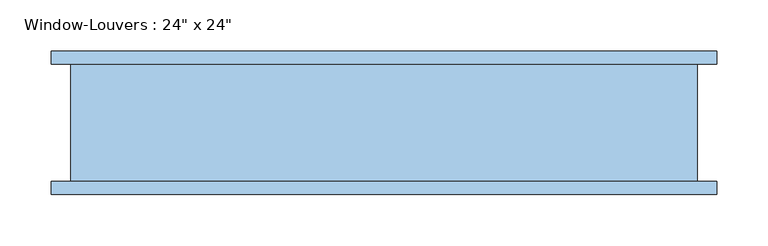
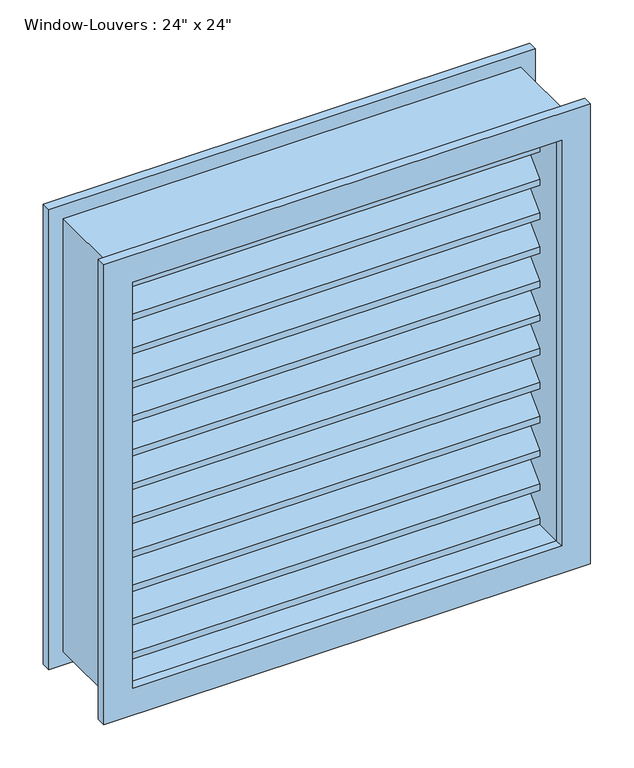
"""IFC4 building model written with IfcOpenShell, lengths in millimetres: window geometry."""

from ifc_helpers import new_model, si_unit, frame, origin, place, context, project, spatial, polyline, outline, extrude, source, transform, mapped, element, save


def window_d39e7ecb(model_context):
    return source(origin(), model_context, "Body", "SweptSolid", [
        extrude(outline(polyline([(50.8, 1419.1754778), (50.8, 1410.1952217), (12.7, 1448.2952217), (-25.4, 1410.1952217), (-25.4, 1419.1754778), (12.7, 1457.2754778), (50.8, 1419.1754778)])), frame((-285.75, 0.0, 0.0), z_axis=(1.0, 0.0, 0.0), x_axis=(0.0, 1.0, 0.0)), (0.0, 0.0, 1.0), 571.5),
        extrude(outline(polyline([(50.8, 1371.5009557), (50.8, 1362.5206995), (12.7, 1400.6206995), (-25.4, 1362.5206995), (-25.4, 1371.5009557), (12.7, 1409.6009557), (50.8, 1371.5009557)])), frame((-285.75, 0.0, 0.0), z_axis=(1.0, 0.0, 0.0), x_axis=(0.0, 1.0, 0.0)), (0.0, 0.0, 1.0), 571.5),
        extrude(outline(polyline([(50.8, 1323.8264335), (50.8, 1314.8461774), (12.7, 1352.9461774), (-25.4, 1314.8461774), (-25.4, 1323.8264335), (12.7, 1361.9264335), (50.8, 1323.8264335)])), frame((-285.75, 0.0, 0.0), z_axis=(1.0, 0.0, 0.0), x_axis=(0.0, 1.0, 0.0)), (0.0, 0.0, 1.0), 571.5),
        extrude(outline(polyline([(50.8, 1276.1519113), (50.8, 1267.1716552), (12.7, 1305.2716552), (-25.4, 1267.1716552), (-25.4, 1276.1519113), (12.7, 1314.2519113), (50.8, 1276.1519113)])), frame((-285.75, 0.0, 0.0), z_axis=(1.0, 0.0, 0.0), x_axis=(0.0, 1.0, 0.0)), (0.0, 0.0, 1.0), 571.5),
        extrude(outline(polyline([(50.8, 1228.4773891), (50.8, 1219.497133), (12.7, 1257.597133), (-25.4, 1219.497133), (-25.4, 1228.4773891), (12.7, 1266.5773891), (50.8, 1228.4773891)])), frame((-285.75, 0.0, 0.0), z_axis=(1.0, 0.0, 0.0), x_axis=(0.0, 1.0, 0.0)), (0.0, 0.0, 1.0), 571.5),
        extrude(outline(polyline([(50.8, 1180.802867), (50.8, 1171.8226109), (12.7, 1209.9226109), (-25.4, 1171.8226109), (-25.4, 1180.802867), (12.7, 1218.902867), (50.8, 1180.802867)])), frame((-285.75, 0.0, 0.0), z_axis=(1.0, 0.0, 0.0), x_axis=(0.0, 1.0, 0.0)), (0.0, 0.0, 1.0), 571.5),
        extrude(outline(polyline([(50.8, 1133.1283448), (50.8, 1124.1480887), (12.7, 1162.2480887), (-25.4, 1124.1480887), (-25.4, 1133.1283448), (12.7, 1171.2283448), (50.8, 1133.1283448)])), frame((-285.75, 0.0, 0.0), z_axis=(1.0, 0.0, 0.0), x_axis=(0.0, 1.0, 0.0)), (0.0, 0.0, 1.0), 571.5),
        extrude(outline(polyline([(50.8, 1085.4538226), (50.8, 1076.4735665), (12.7, 1114.5735665), (-25.4, 1076.4735665), (-25.4, 1085.4538226), (12.7, 1123.5538226), (50.8, 1085.4538226)])), frame((-285.75, 0.0, 0.0), z_axis=(1.0, 0.0, 0.0), x_axis=(0.0, 1.0, 0.0)), (0.0, 0.0, 1.0), 571.5),
        extrude(outline(polyline([(50.8, 1037.7793005), (50.8, 1028.7990443), (12.7, 1066.8990443), (-25.4, 1028.7990443), (-25.4, 1037.7793005), (12.7, 1075.8793005), (50.8, 1037.7793005)])), frame((-285.75, 0.0, 0.0), z_axis=(1.0, 0.0, 0.0), x_axis=(0.0, 1.0, 0.0)), (0.0, 0.0, 1.0), 571.5),
        extrude(outline(polyline([(50.8, 990.1047783), (50.8, 981.1245222), (12.7, 1019.2245222), (-25.4, 981.1245222), (-25.4, 990.1047783), (12.7, 1028.2047783), (50.8, 990.1047783)])), frame((-285.75, 0.0, 0.0), z_axis=(1.0, 0.0, 0.0), x_axis=(0.0, 1.0, 0.0)), (0.0, 0.0, 1.0), 571.5),
        extrude(outline(polyline([(50.8, 1466.85), (50.8, 1457.8697439), (12.7, 1495.9697439), (-25.4, 1457.8697439), (-25.4, 1466.85), (12.7, 1504.95), (50.8, 1466.85)])), frame((-285.75, 0.0, 0.0), z_axis=(1.0, 0.0, 0.0), x_axis=(0.0, 1.0, 0.0)), (0.0, 0.0, 1.0), 571.5),
        extrude(outline(polyline([(50.8, 942.4302561), (50.8, 933.45), (12.7, 971.55), (-25.4, 933.45), (-25.4, 942.4302561), (12.7, 980.5302561), (50.8, 942.4302561)])), frame((-285.75, 0.0, 0.0), z_axis=(1.0, 0.0, 0.0), x_axis=(0.0, 1.0, 0.0)), (0.0, 0.0, 1.0), 571.5),
        extrude(outline(polyline([(1524.0, 304.8), (1524.0, -304.8), (914.4, -304.8), (914.4, 304.8), (1524.0, 304.8)]), holes=[polyline([(1504.95, 285.75), (933.45, 285.75), (933.45, -285.75), (1504.95, -285.75), (1504.95, 285.75)])]), frame((0.0, -63.5, 0.0), z_axis=(0.0, 1.0, 0.0), x_axis=(0.0, 0.0, 1.0)), (0.0, 0.0, 1.0), 114.3),
        extrude(outline(polyline([(1543.05, 323.85), (1543.05, -323.85), (895.35, -323.85), (895.35, 323.85), (1543.05, 323.85)]), holes=[polyline([(1504.95, 285.75), (933.45, 285.75), (933.45, -285.75), (1504.95, -285.75), (1504.95, 285.75)])]), frame((0.0, -76.2, 0.0), z_axis=(0.0, 1.0, 0.0), x_axis=(0.0, 0.0, 1.0)), (0.0, 0.0, 1.0), 12.7),
        extrude(outline(polyline([(1543.05, -323.85), (895.35, -323.85), (895.35, 323.85), (1543.05, 323.85), (1543.05, -323.85)]), holes=[polyline([(1504.95, -285.75), (1504.95, 285.75), (933.45, 285.75), (933.45, -285.75), (1504.95, -285.75)])]), frame((0.0, 50.8, 0.0), z_axis=(0.0, 1.0, 0.0), x_axis=(0.0, 0.0, 1.0)), (0.0, 0.0, 1.0), 12.7),
    ])


if __name__ == "__main__":
    model = new_model("IFC4")
    model_context = context("Model", 3, world=origin())
    ifc_project = project(units=[si_unit("LENGTHUNIT", "METRE", prefix="MILLI")], contexts=[model_context])
    site = spatial("IfcSite", under=ifc_project)
    building = spatial("IfcBuilding", under=site)
    placement = place(None, origin())
    window_shape = window_d39e7ecb(model_context)
    element("IfcWindow", 1, ObjectType="Window-Louvers : 24\" x 24\"", at=placement, inside=building, context=model_context, shape_type="MappedRepresentation", body=[
        mapped(window_shape, transform((0.0, 0.0, 0.0), x_axis=(1.0, 0.0, 0.0), y_axis=(0.0, 1.0, 0.0), z_axis=(0.0, 0.0, 1.0))),
    ])
    save(model, "model.ifc")

# Revit data of these elements
# Type "Window-Louvers : 24\" x 24\""
#   Type Mark = "20"
#   Construction Type Id = "GSP4R"
#   Assembly Code = "B20"
#   Analytic Construction = "1/8 in Pilkington single glazing"
#   Visual Light Transmittance = 0.9
#   Thermal Resistance (R) = 1.53941 (h·ft²·°F)/BTU
#   Solar Heat Gain Coefficient = 0.78
#   Max Height = 1' - 11.74264"
#   Height = 2' - 0"
#   Heat Transfer Coefficient (U) = 0.6496 BTU/(h·ft²·°F)
#   Blade Width [instance default] = 1' - 10 1/2"
#   Blade Vertical Thickness = 0' - 0.35355"
#   Blade Thickness = 0' - 0 1/4"
#   Blade Spacing = 0' - 1 1/2"
#   Blade Height = 0' - 1.85355"
#   Blade Depth = 0' - 3"
#   Blade Angle = 45.00°
#   Default Sill Height = 3' - 0"
#   Trim Projection_Exterior = 0' - 0 1/2"
#   Trim Projection_Interior = 0' - 0 1/2"
#   Trim Width_Exterior = 0' - 1 1/2"
#   Trim Width_Interior = 0' - 1 1/2"
#   Width = 2' - 0"
#   Max Blade Count = 12
#   Define Thermal Properties by = 1
#   Blade Count = 12
#   Frame Material = Birch
#   Louver Material = Birch
#   Trim Exterior Material = Birch
#   Trim Interior Material = Birch
#   Wall Closure = (empty or 0)
# Element 1 (IfcWindow, "Window-Louvers : 24\" x 24\"")
#   Materials on its faces: "Birch"
# Materials
#   "Birch": class "Wood", colour RGB 224 178 126, transparency 0, Description = "Betula Alleghaniensis", Cost = 0
